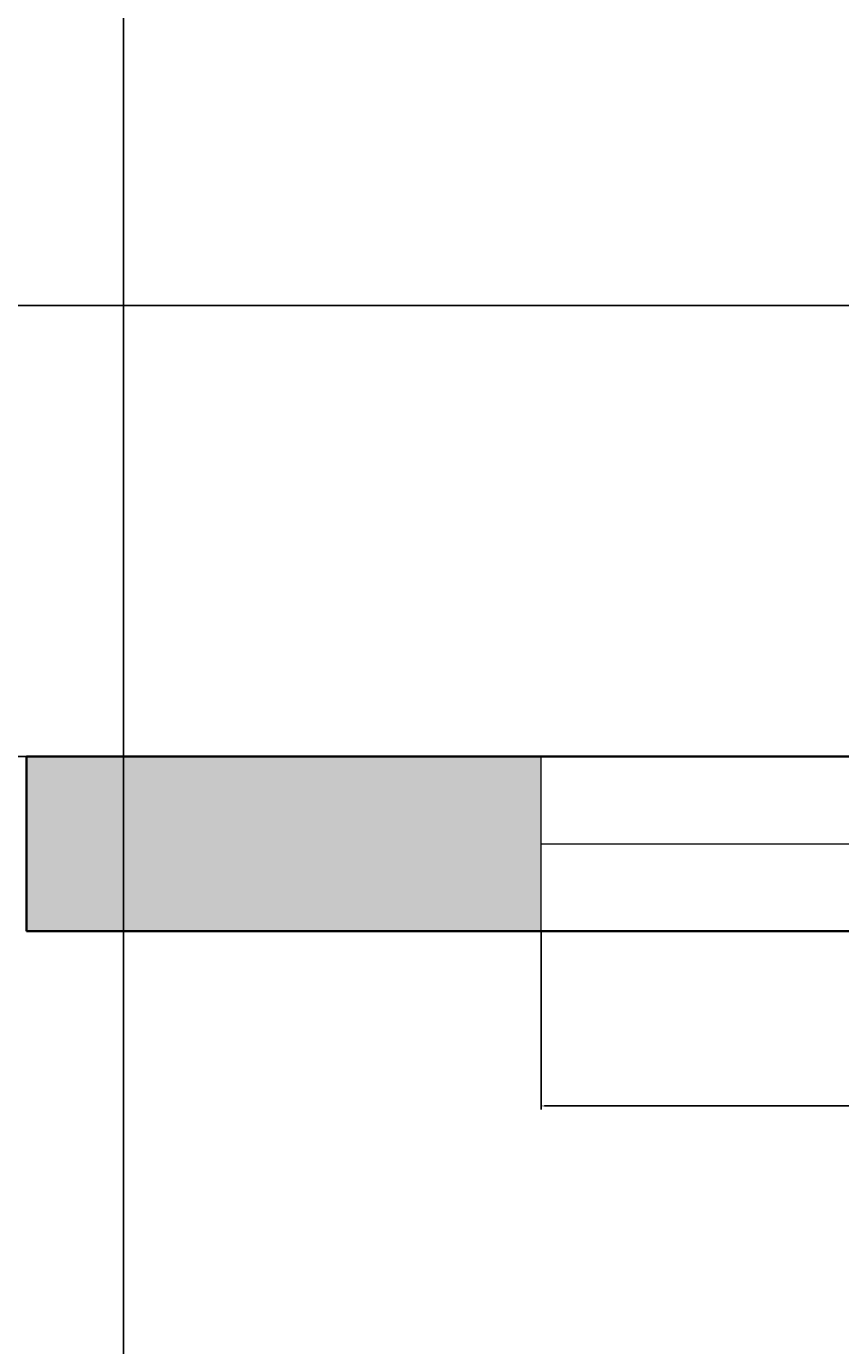
# Model space of a CAD drawing. Units: inches. Extents: x -5 to 330, y -522 to 40.
# Tile 14 of 23: x 159 to 201, y -447 to -380. Entities that reach past the tile are written whole.
import ezdxf

# ---------------------------------------------------------------- set-up
doc = ezdxf.new("R2010")
doc.units = ezdxf.units.IN
doc.header["$MEASUREMENT"] = 0
for name, color, linetype, lineweight in [('A-ANNO-DIMS', 2, 'Continuous', 18), ('A-GLAZ', 4, 'Continuous', 18), ('A-WALL', 7, 'Continuous', 35)]:
    doc.layers.add(name, color=color, linetype=linetype, lineweight=lineweight)
doc.layers.add('A-WALL-PATT', color=18, linetype='Continuous', lineweight=13, true_color=0x000000)
doc.styles.get("Standard").update_dxf_attribs({"font": 'arial.ttf'})
doc.dimstyles.get("Standard").update_dxf_attribs({"dimtxt": 0.18, "dimasz": 0.18, "dimexe": 0.18, "dimexo": 0.0625, "dimgap": 0.09, "dimtad": 0, "dimtih": 1, "dimtoh": 1, "dimdec": 0, "dimzin": 0, "dimdsep": 46, "dimlunit": 3, "dimtxsty": 'Standard', "dimcen": 0.09, "dimadec": 0, "dimazin": 0, "dimtfac": 1, "dimtdec": 0, "dimtofl": 0, "dimtmove": 0, "dimatfit": 3, "dimfxl": 1, "dimtolj": 1, "dimtzin": 0, "dimarcsym": 0})

# ---------------------------------------------------------------- blocks, each defined once
blk = doc.blocks.new('WIN-60IN-GLAZ')
for p, q in [((0, 9), (60, 9)), ((0, 4.5), (60, 4.5)), ((60, 0), (0, 0))]:
    blk.add_line(p, q)
blk = doc.blocks.new('*D19')
at = {"layer": 'A-ANNO-DIMS', "color": 0, "lineweight": -2, "transparency": 16777216}
for p, q in [((185.51, -426.206), (185.51, -435.324)), ((245.51, -426.206), (245.51, -435.324)), ((185.69, -435.144), (214.281, -435.144)), ((245.33, -435.144), (216.739, -435.144))]:
    blk.add_line(p, q, dxfattribs=at)
at = {"layer": 'A-ANNO-DIMS', "color": 0, "transparency": 16777216}
for points in [[(185.69, -435.114), (185.69, -435.174), (185.51, -435.144)], [(245.33, -435.114), (245.33, -435.174), (245.51, -435.144)]]:
    blk.add_solid(points, dxfattribs=at)
at = {"layer": 'Defpoints', "color": 0, "transparency": 16777216}
for p in [(185.51, -426.144), (245.51, -426.144), (245.51, -435.144)]:
    blk.add_point(p, dxfattribs=at)
at = {"layer": 'A-ANNO-DIMS', "color": 0, "transparency": 16777216, "insert": (215.51, -435.144), "char_height": 0.18, "attachment_point": 5}
blk.add_mtext('\\A1;WINDOW 5\'-0" TYP.', dxfattribs=at)
blk = doc.blocks.new('*D37')
at = {"layer": 'A-ANNO-DIMS', "color": 0, "lineweight": -2, "transparency": 16777216}
for p, q in [((164.01, -53.206), (164.01, -522.309)), ((272.01, -53.206), (272.01, -522.309)), ((164.19, -522.129), (217.681, -522.129)), ((271.83, -522.129), (218.339, -522.129))]:
    blk.add_line(p, q, dxfattribs=at)
at = {"layer": 'A-ANNO-DIMS', "color": 0, "transparency": 16777216}
for points in [[(164.19, -522.099), (164.19, -522.159), (164.01, -522.129)], [(271.83, -522.099), (271.83, -522.159), (272.01, -522.129)]]:
    blk.add_solid(points, dxfattribs=at)
at = {"layer": 'Defpoints', "color": 0, "transparency": 16777216}
for p in [(164.01, -53.144), (272.01, -53.144), (272.01, -522.129)]:
    blk.add_point(p, dxfattribs=at)
at = {"layer": 'A-ANNO-DIMS', "color": 0, "transparency": 16777216, "insert": (218.01, -522.129), "char_height": 0.18, "attachment_point": 5}
blk.add_mtext('\\A1;9\'-0"', dxfattribs=at)
blk = doc.blocks.new('*D44')
at = {"layer": 'A-ANNO-DIMS', "color": 0, "lineweight": -2, "transparency": 16777216}
for p, q in [((128.572, -393.928), (308.175, -393.928)), ((307.995, -394.108), (307.995, -405.356)), ((307.995, -416.964), (307.995, -405.716)), ((128.572, -417.144), (308.175, -417.144))]:
    blk.add_line(p, q, dxfattribs=at)
at = {"layer": 'A-ANNO-DIMS', "color": 0, "transparency": 16777216}
for points in [[(307.965, -394.108), (308.025, -394.108), (307.995, -393.928)], [(307.965, -416.964), (308.025, -416.964), (307.995, -417.144)]]:
    blk.add_solid(points, dxfattribs=at)
at = {"layer": 'Defpoints', "color": 0, "transparency": 16777216}
for p in [(128.51, -393.928), (307.995, -393.928), (128.51, -417.144)]:
    blk.add_point(p, dxfattribs=at)
at = {"layer": 'A-ANNO-DIMS', "color": 0, "transparency": 16777216, "insert": (307.995, -405.536), "char_height": 0.18, "attachment_point": 5}
blk.add_mtext('\\A1;1\'-11"', dxfattribs=at)

msp = doc.modelspace()

# ---------------------------------------------------------------- hatches: boundary and pattern name
at = {"layer": 'A-WALL-PATT'}
h = msp.add_hatch(color=256, dxfattribs=at)
h.dxf.hatch_style = 1
h.paths.add_polyline_path([(164.01, -44.152), (159.51, -44.152), (159.51, -153.144), (164.01, -153.144)], flags=17)
h.paths.add_polyline_path([(224.01, -188.144), (272.01, -188.144), (272.01, -218.144), (260.01, -218.144), (260.01, -222.644), (272.01, -222.644), (272.01, -292.644), (159.01, -292.644), (159.01, -297.144), (272.01, -297.144), (272.01, -417.144), (245.51, -417.144), (245.51, -426.144), (272.01, -426.144), (272.01, -495.144), (281.01, -495.144), (281.01, 12.356), (23.51, 12.356), (23.51, -426.144), (62.918, -426.144), (62.918, -417.144), (32.51, -417.144), (32.51, -297.144), (48.129, -297.144), (48.129, -292.644), (32.51, -292.644), (32.51, -140.644), (133.51, -140.644), (133.51, -131.644), (32.51, -131.644), (32.51, 3.356), (159.51, 3.356), (164.01, 3.356), (220.01, 3.356), (224.51, 3.356), (272.01, 3.356), (272.01, -179.144), (159.51, -179.144), (159.51, -188.144), (219.51, -188.144), (219.51, -266.644), (224.01, -266.644), (224.01, -222.644), (236.01, -222.644), (236.01, -218.144), (224.01, -218.144)])
h.paths.add_polyline_path([(133.01, -292.644), (128.51, -292.644), (128.51, -297.144), (128.51, -417.144), (122.918, -417.144), (122.918, -426.144), (133.01, -426.144)], flags=17)
h.paths.add_polyline_path([(185.51, -417.144), (159.01, -417.144), (159.01, -426.144), (185.51, -426.144)], flags=17)
h.paths.add_polyline_path([(133.51, -140.644), (129.01, -140.644), (129.01, -246.644), (133.51, -246.644)], flags=17)
h.paths.add_polyline_path([(246.01, -48.644), (224.51, -48.644), (224.51, -27.627), (220.01, -27.627), (220.01, -48.644), (198.604, -48.644), (198.604, -53.144), (246.01, -53.144)], flags=17)

# ---------------------------------------------------------------- linework, layer by layer
at = {"layer": 'A-GLAZ'}
msp.add_line((185.51, -426.144), (185.51, -417.144), dxfattribs=at)
at = {"layer": 'A-WALL'}
for p, q in [((159.01, -417.144), (159.01, -426.144)), ((159.01, -417.144), (272.01, -417.144)), ((159.01, -426.144), (272.01, -426.144))]:
    msp.add_line(p, q, dxfattribs=at)

# ---------------------------------------------------------------- block references
at = {"layer": 'A-GLAZ'}
msp.add_blockref('WIN-60IN-GLAZ', (185.51, -426.144), dxfattribs=at)

# ---------------------------------------------------------------- dimensions: what is measured, and where the dimension line sits
at = {"layer": 'A-ANNO-DIMS'}
dim = msp.add_linear_dim(base=(272.01, -522.129), p1=(164.01, -53.144), p2=(272.01, -53.144), dimstyle='Standard', override={"dimdec": 1, "dimlfac": 1, "dimrnd": 0, "dimzin": 1, "dimdsep": 46, "dimlunit": 4, "dimfrac": 2}, dxfattribs=at)
dim.commit()
dim.dimension.update_dxf_attribs({"geometry": '*D37', "text_midpoint": (218.01, -522.129)})
dim = msp.add_linear_dim(base=(307.995, -393.928), p1=(128.51, -417.144), p2=(128.51, -393.928), angle=90, dimstyle='Standard', override={"dimdec": 1, "dimlfac": 1, "dimrnd": 0, "dimzin": 1, "dimdsep": 46, "dimlunit": 4, "dimfrac": 2}, dxfattribs=at)
dim.commit()
dim.dimension.update_dxf_attribs({"geometry": '*D44', "text_midpoint": (307.995, -405.536)})
dim = msp.add_linear_dim(base=(245.51, -435.144), p1=(185.51, -426.144), p2=(245.51, -426.144), text='WINDOW <> TYP.', dimstyle='Standard', override={"dimdec": 1, "dimlfac": 1, "dimrnd": 0, "dimzin": 1, "dimdsep": 46, "dimlunit": 4, "dimfrac": 2}, dxfattribs=at)
dim.commit()
dim.dimension.update_dxf_attribs({"geometry": '*D19', "text_midpoint": (215.51, -435.144)})

doc.saveas('drawing.dxf')
